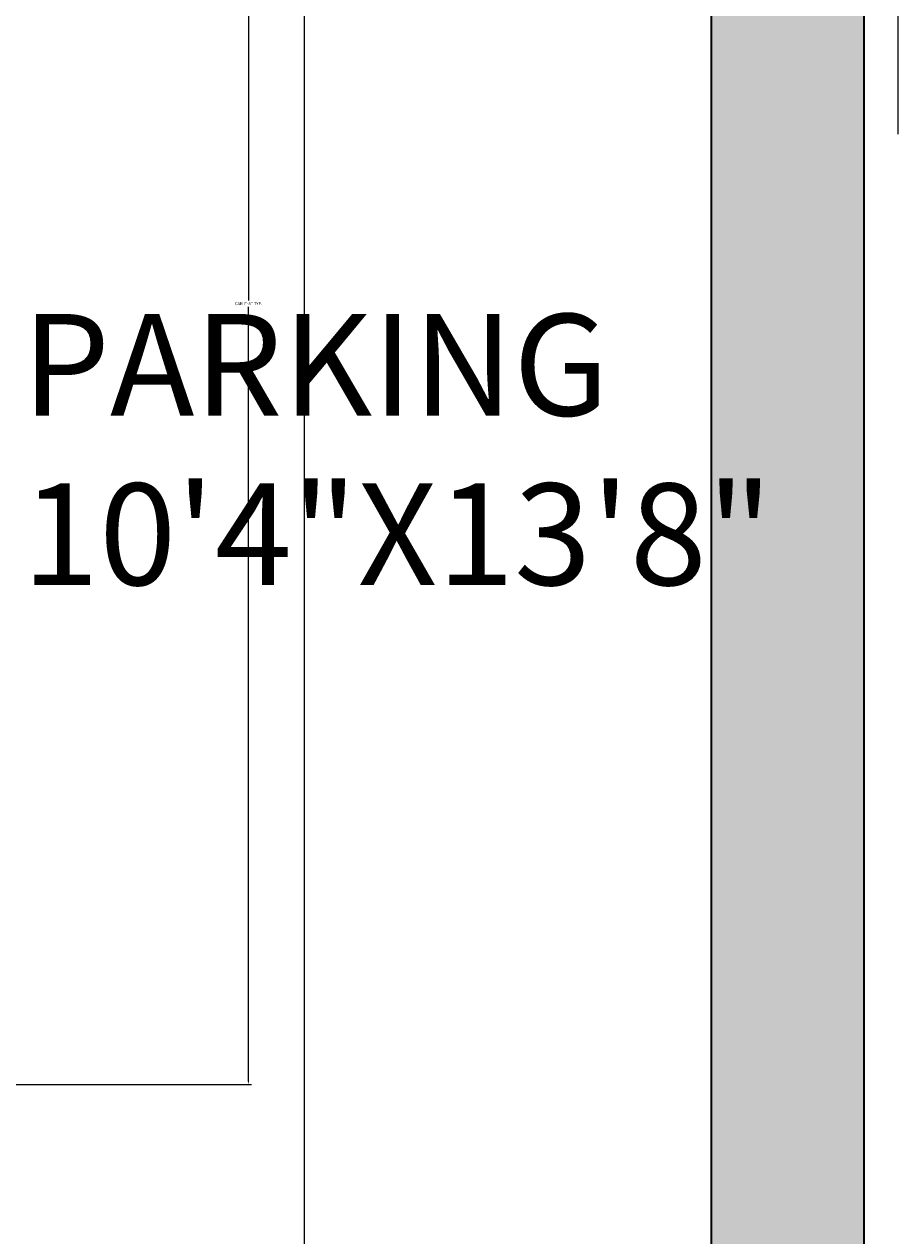
# Model space of a CAD drawing. Units: inches. Extents: x 37 to 706, y -568 to 110.
# Tile 5 of 24: x 171 to 223, y -450 to -378. Entities that reach past the tile are written whole.
import ezdxf

# ---------------------------------------------------------------- set-up
doc = ezdxf.new("R2010")
doc.units = ezdxf.units.IN
doc.header["$MEASUREMENT"] = 0
for name, color, linetype, lineweight in [('A-ANNO-DIMS', 2, 'Continuous', 18), ('A-AREA-IDEN', 7, 'Continuous', 18), ('A-DOOR', 4, 'Continuous', 18), ('A-WALL', 7, 'Continuous', 35), ('A-WALL-PATT', 252, 'Continuous', 13)]:
    doc.layers.add(name, color=color, linetype=linetype, lineweight=lineweight)
doc.styles.get("Standard").update_dxf_attribs({"font": 'arial.ttf'})
doc.dimstyles.get("Standard").update_dxf_attribs({"dimtxt": 0.18, "dimasz": 0.18, "dimexe": 0.18, "dimexo": 0.0625, "dimgap": 0.09, "dimtad": 0, "dimtih": 1, "dimtoh": 1, "dimdec": 0, "dimzin": 0, "dimdsep": 46, "dimlunit": 3, "dimtxsty": 'Standard', "dimcen": 0.09, "dimadec": 0, "dimazin": 0, "dimtfac": 1, "dimtdec": 0, "dimtofl": 0, "dimtmove": 0, "dimatfit": 3, "dimfxl": 1, "dimtolj": 1, "dimtzin": 0, "dimarcsym": 0})

# ---------------------------------------------------------------- blocks, each defined once
blk = doc.blocks.new('*D29')
at = {"layer": 'A-ANNO-DIMS', "color": 0, "lineweight": -2, "transparency": 16777216}
for p, q in [((170.913, -348.62), (184.856, -348.62)), ((184.676, -348.8), (184.676, -394.522)), ((184.676, -440.609), (184.676, -394.888)), ((170.913, -440.789), (184.856, -440.789))]:
    blk.add_line(p, q, dxfattribs=at)
at = {"layer": 'A-ANNO-DIMS', "color": 0, "transparency": 16777216}
for points in [[(184.646, -348.8), (184.706, -348.8), (184.676, -348.62)], [(184.646, -440.609), (184.706, -440.609), (184.676, -440.789)]]:
    blk.add_solid(points, dxfattribs=at)
at = {"layer": 'Defpoints', "color": 0, "transparency": 16777216}
for p in [(170.851, -348.62), (184.676, -348.62), (170.851, -440.789)]:
    blk.add_point(p, dxfattribs=at)
at = {"layer": 'A-ANNO-DIMS', "color": 0, "transparency": 16777216, "insert": (184.676, -394.705), "char_height": 0.18, "attachment_point": 5}
blk.add_mtext('\\A1;CAR 7\'-8" TYP.', dxfattribs=at)
blk = doc.blocks.new('*D51')
at = {"layer": 'A-ANNO-DIMS', "color": 0, "lineweight": -2, "transparency": 16777216}
for p, q in [((220.958, -294.771), (220.958, -567.638)), ((251.958, -294.771), (251.958, -567.638)), ((221.138, -567.458), (236.128, -567.458)), ((251.778, -567.458), (236.789, -567.458))]:
    blk.add_line(p, q, dxfattribs=at)
at = {"layer": 'A-ANNO-DIMS', "color": 0, "transparency": 16777216}
for points in [[(221.138, -567.428), (221.138, -567.488), (220.958, -567.458)], [(251.778, -567.428), (251.778, -567.488), (251.958, -567.458)]]:
    blk.add_solid(points, dxfattribs=at)
at = {"layer": 'Defpoints', "color": 0, "transparency": 16777216}
for p in [(220.958, -294.708), (251.958, -294.708), (251.958, -567.458)]:
    blk.add_point(p, dxfattribs=at)
at = {"layer": 'A-ANNO-DIMS', "color": 0, "transparency": 16777216, "insert": (236.458, -567.458), "char_height": 0.18, "attachment_point": 5}
blk.add_mtext('\\A1;2\'-7"', dxfattribs=at)
blk = doc.blocks.new('*D62')
at = {"layer": 'A-ANNO-DIMS', "color": 0, "lineweight": -2, "transparency": 16777216}
for p, q in [((187.958, -142.771), (187.958, -567.638)), ((211.958, -142.771), (211.958, -567.638)), ((188.138, -567.458), (199.628, -567.458)), ((211.778, -567.458), (200.289, -567.458))]:
    blk.add_line(p, q, dxfattribs=at)
at = {"layer": 'A-ANNO-DIMS', "color": 0, "transparency": 16777216}
for points in [[(188.138, -567.428), (188.138, -567.488), (187.958, -567.458)], [(211.778, -567.428), (211.778, -567.488), (211.958, -567.458)]]:
    blk.add_solid(points, dxfattribs=at)
at = {"layer": 'Defpoints', "color": 0, "transparency": 16777216}
for p in [(187.958, -142.708), (211.958, -142.708), (211.958, -567.458)]:
    blk.add_point(p, dxfattribs=at)
at = {"layer": 'A-ANNO-DIMS', "color": 0, "transparency": 16777216, "insert": (199.958, -567.458), "char_height": 0.18, "attachment_point": 5}
blk.add_mtext('\\A1;2\'-0"', dxfattribs=at)

msp = doc.modelspace()

# ---------------------------------------------------------------- hatches: boundary and pattern name
at = {"layer": 'A-WALL-PATT'}
h = msp.add_hatch(color=256, dxfattribs=at)
h.dxf.hatch_style = 1
h.paths.add_polyline_path([(220.958, -351.708), (211.958, -351.708), (211.958, -513.708), (254.958, -513.708), (254.958, -504.708), (220.958, -504.708)], flags=17)
h.paths.add_polyline_path([(220.958, -294.708), (211.958, -294.708), (211.958, -303.708), (220.958, -303.708)], flags=17)
h.paths.add_polyline_path([(175.958, -294.708), (155.871, -294.708), (155.871, -303.708), (155.958, -303.708), (175.958, -303.708)], flags=17)
h.paths.add_polyline_path([(220.958, -16.708), (211.958, -16.708), (211.958, -142.708), (220.958, -142.708)], flags=17)
h.paths.add_polyline_path([(357.958, 51.292), (78.958, 51.292), (78.958, -513.708), (87.958, -513.708), (87.958, -303.708), (95.871, -303.708), (95.871, -294.708), (87.958, -294.708), (87.958, -142.708), (187.958, -142.708), (187.958, -133.708), (87.958, -133.708), (87.958, -25.708), (106.958, -25.708), (106.958, -16.708), (87.958, -16.708), (87.958, 42.292), (348.958, 42.292), (348.958, 17.129), (348.958, -133.708), (246.958, -133.708), (246.958, -142.708), (348.958, -142.708), (348.958, -294.708), (251.958, -294.708), (251.958, -303.708), (348.958, -303.708), (348.958, -351.708), (260.958, -351.708), (260.958, -329.708), (251.958, -329.708), (251.958, -360.708), (327.446, -360.708), (348.958, -360.708), (348.958, -504.708), (314.958, -504.708), (314.958, -513.708), (357.958, -513.708)])
h.paths.add_polyline_path([(416.958, -303.708), (402.958, -303.708), (402.958, -151.708), (478.958, -151.708), (478.958, -142.708), (402.958, -142.708), (402.958, -22.708), (409.958, -22.708), (409.958, -13.708), (402.958, -13.708), (402.958, 42.292), (663.958, 42.292), (663.958, -303.708), (566.958, -303.708), (566.958, -312.708), (663.958, -312.708), (663.958, -360.708), (575.958, -360.708), (575.958, -338.708), (566.958, -338.708), (566.958, -360.708), (566.958, -369.708), (642.446, -369.708), (663.958, -369.708), (663.958, -513.708), (629.958, -513.708), (629.958, -522.708), (672.958, -522.708), (672.958, 51.292), (393.958, 51.292), (393.958, -522.708), (402.958, -522.708), (402.958, -312.708), (416.958, -312.708)])
h.paths.add_polyline_path([(490.958, -303.708), (476.958, -303.708), (476.958, -312.708), (490.958, -312.708)], flags=17)
h.paths.add_polyline_path([(535.958, -303.708), (526.958, -303.708), (526.958, -312.708), (535.958, -312.708)], flags=17)
h.paths.add_polyline_path([(535.958, -369.708), (526.958, -369.708), (526.958, -522.708), (569.958, -522.708), (569.958, -513.708), (535.958, -513.708)], flags=17)
h.paths.add_polyline_path([(511.958, -13.708), (502.958, -13.708), (502.958, -151.708), (511.958, -151.708)], flags=17)
h.paths.add_polyline_path([(651.539, -142.708), (651.539, -120.181), (642.539, -120.181), (642.539, -142.708), (550.539, -142.708), (550.539, -120.708), (541.539, -120.708), (541.539, -142.708), (537.958, -142.708), (537.958, -151.708), (651.539, -151.708)], flags=17)
h.paths.add_polyline_path([(651.539, -85.708), (541.539, -85.708), (541.539, -94.708), (651.539, -94.708)], flags=17)
h.paths.add_polyline_path([(476.958, -13.708), (469.958, -13.708), (469.958, -22.708), (476.958, -22.708)], flags=17)
h.paths.add_polyline_path([(185.958, -16.708), (166.958, -16.708), (166.958, -25.708), (185.958, -25.708)], flags=17)
h.paths.add_polyline_path([(168.909, -414.719), (214.621, -414.719), (214.621, -392.33), (168.909, -392.33)], flags=25)

# ---------------------------------------------------------------- linework, layer by layer
at = {"layer": 'A-DOOR'}
msp.add_line((222.958, -360.708), (222.958, -384.708), dxfattribs=at)
at = {"layer": 'A-WALL'}
for p, q in [((211.958, -294.708), (211.958, -513.708)), ((220.958, -294.708), (220.958, -504.708))]:
    msp.add_line(p, q, dxfattribs=at)

# ---------------------------------------------------------------- texts
at = {"layer": 'A-AREA-IDEN', "insert": (171.322, -395.316), "char_height": 6, "attachment_point": 1}
msp.add_mtext('PARKING\\P10\'4"X13\'8"', dxfattribs=at)

# ---------------------------------------------------------------- dimensions: what is measured, and where the dimension line sits
at = {"layer": 'A-ANNO-DIMS'}
for base, p1, p2, picture, middle in [((211.958, -567.458), (187.958, -142.708), (211.958, -142.708), '*D62', (199.958, -567.458)), ((251.958, -567.458), (220.958, -294.708), (251.958, -294.708), '*D51', (236.458, -567.458))]:
    dim = msp.add_linear_dim(base=base, p1=p1, p2=p2, dimstyle='Standard', override={"dimdec": 1, "dimlfac": 1, "dimrnd": 0, "dimzin": 1, "dimdsep": 46, "dimlunit": 4, "dimfrac": 2}, dxfattribs=at)
    dim.commit()
    dim.dimension.update_dxf_attribs({"geometry": picture, "text_midpoint": middle})
dim = msp.add_linear_dim(base=(184.676, -348.62), p1=(170.851, -440.789), p2=(170.851, -348.62), angle=90, text='CAR <> TYP.', dimstyle='Standard', override={"dimdec": 1, "dimlfac": 1, "dimrnd": 0, "dimzin": 1, "dimdsep": 46, "dimlunit": 4, "dimfrac": 2}, dxfattribs=at)
dim.commit()
dim.dimension.update_dxf_attribs({"geometry": '*D29', "text_midpoint": (184.676, -394.705)})

doc.saveas('drawing.dxf')
